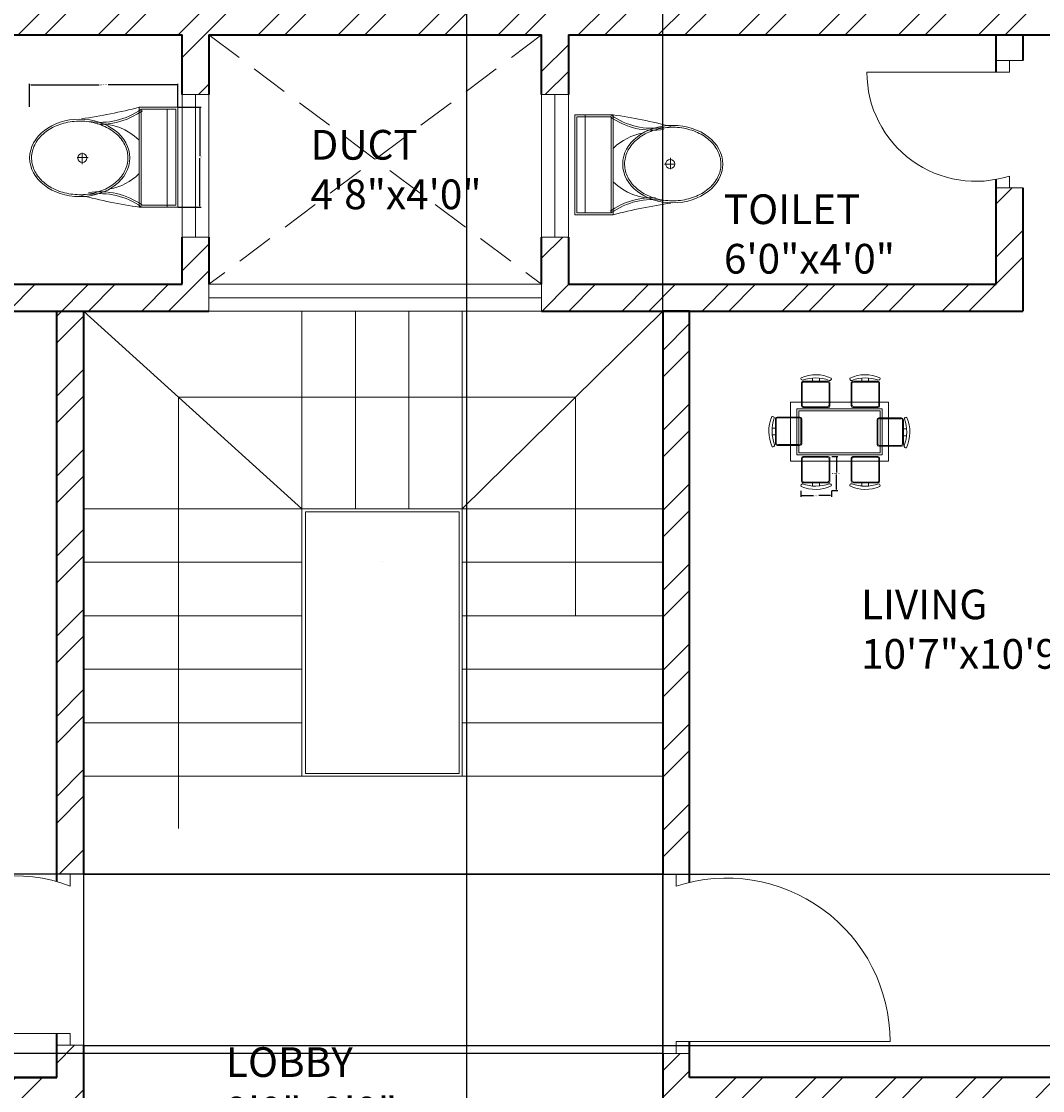
# Model space of a CAD drawing. Units: inches. Extents: x 1570 to 2186, y 1575 to 2421.
# Tile 8 of 10: x 1806 to 1978, y 2045 to 2225. Entities that reach past the tile are written whole.
import ezdxf

# ---------------------------------------------------------------- set-up
doc = ezdxf.new("R2010")
doc.units = ezdxf.units.IN
doc.linetypes.add('DASHED2', pattern=[9.525, 6.35, -3.175])
for name, color, linetype, lineweight in [('A-ANNO-DIMS', 2, 'Continuous', 18), ('A-AREA-IDEN', 7, 'Continuous', 18), ('A-DOOR', 201, 'Continuous', 18), ('A-FLOR-FIXT', 9, 'Continuous', 18), ('A-FLOR-OPEN', 254, 'DASHED2', 13), ('A-FLOR-STRS', 201, 'Continuous', 18), ('A-FURN', 8, 'Continuous', 13), ('A-GLAZ', 150, 'Continuous', 18), ('A-WALL', 7, 'Continuous', 35), ('A-WALL-PATT', 252, 'Continuous', 13)]:
    doc.layers.add(name, color=color, linetype=linetype, lineweight=lineweight)
doc.styles.get("Standard").update_dxf_attribs({"font": 'arial.ttf'})
doc.dimstyles.get("Standard").update_dxf_attribs({"dimtxt": 0.18, "dimasz": 0.18, "dimexe": 0.18, "dimexo": 0.0625, "dimgap": 0.09, "dimtad": 0, "dimtih": 1, "dimtoh": 1, "dimdec": 4, "dimzin": 0, "dimdsep": 46, "dimtxsty": 'Standard', "dimcen": 0.09, "dimadec": 0, "dimazin": 0, "dimtfac": 1, "dimtdec": 4, "dimtofl": 0, "dimtmove": 0, "dimatfit": 3, "dimfxl": 1, "dimtolj": 1, "dimtzin": 0, "dimarcsym": 0})

# ---------------------------------------------------------------- blocks, each defined once
blk = doc.blocks.new('A$C31115884')
for p, q in [((257.5, 466.4), (257.5, 523.2)), ((283.1, 497.7), (223.4, 497.7)), ((0, 200), (0, 0)), ((520, 200), (0, 200)), ((10, 190), (10, 10)), ((510, 190), (10, 190)), ((510, 10), (510, 190)), ((520, 0), (520, 200)), ((510, 54.5), (0, 54.5)), ((10, 10), (510, 10)), ((0, 0), (520, 0))]:
    blk.add_line(p, q)
blk.add_circle((255.6, 496.4), 23.6)
for centre, radius, start, end in [((2777.7, -204.6), 2807, 165.4549, 171.7133), ((-294.5, 403.3), 364.7, 324.2091, 9.3499), ((-294.5, 403.3), 374.7, 324.2091, 9.3499), ((805.8, 403.3), 364.7, 170.6501, 215.7909), ((3237, 905), 2807, 188.2867, 194.5451), ((139.5, 406.2), 293.5, 315.8436, 2.6563), ((805.8, 403.3), 374.7, 179.2036, 215.7909), ((383.6, 406.2), 293.5, 190.2774, 224.1564)]:
    blk.add_arc(centre, radius, start, end)
blk.add_ellipse((256.2, 509.9), major_axis=(0, -260.7), ratio=0.772727)
blk.add_open_spline([(256.2, 259.2), (263.1, 259.2), (270, 259.7), (287.8, 262.3), (298.7, 265.1), (319.9, 273.1), (330.2, 278.4), (350.1, 291.1), (359.7, 298.7), (377.7, 315.9), (386.2, 325.5), (401.7, 346.6), (408.8, 358.1), (421.3, 382.5), (426.8, 395.5), (435.9, 422.4), (439.5, 436.4), (444.8, 465.1), (446.5, 479.7), (447.9, 509.2), (447.6, 524), (445, 553.3), (442.7, 567.8), (436.3, 596), (432.1, 609.7), (421.9, 636), (416, 648.6), (402.5, 672.1), (395, 683), (378.6, 703), (369.8, 712.1), (351.1, 728), (341.3, 734.8), (320.9, 746.2), (310.4, 750.7), (288.9, 757.3), (278, 759.4), (256, 761), (245, 760.6), (223.1, 757.2), (212.3, 754.3), (191.1, 746.1), (180.8, 740.7), (160.9, 727.8), (151.4, 720.1), (133.5, 702.7), (125.1, 693), (109.6, 671.7), (102.6, 660.2), (90.2, 635.7), (84.9, 622.7), (76, 595.6), (72.4, 581.6), (67.2, 552.9), (65.6, 538.2), (64.4, 508.8), (64.8, 494), (67.5, 464.7), (69.9, 450.2), (76.6, 422), (80.8, 408.3), (91.1, 382.2), (97.2, 369.7), (110.8, 346.3), (118.4, 335.4), (134.8, 315.6), (143.7, 306.7), (162.4, 290.9), (172.3, 284.2), (192.8, 273), (203.3, 268.6), (224.8, 262.2), (235.8, 260.2), (249.9, 259.3), (253, 259.2), (256.2, 259.2)], degree=3, knots=[0, 0, 0, 0, 0.110105, 0.110105, 0.285049, 0.285049, 0.459994, 0.459994, 0.634938, 0.634938, 0.809882, 0.809882, 0.984827, 0.984827, 1.159771, 1.159771, 1.334715, 1.334715, 1.50966, 1.50966, 1.684604, 1.684604, 1.859549, 1.859549, 2.034493, 2.034493, 2.209437, 2.209437, 2.384382, 2.384382, 2.559326, 2.559326, 2.73427, 2.73427, 2.909215, 2.909215, 3.084159, 3.084159, 3.259103, 3.259103, 3.434048, 3.434048, 3.608992, 3.608992, 3.783936, 3.783936, 3.958881, 3.958881, 4.133825, 4.133825, 4.30877, 4.30877, 4.483714, 4.483714, 4.658658, 4.658658, 4.833603, 4.833603, 5.008547, 5.008547, 5.183491, 5.183491, 5.358436, 5.358436, 5.53338, 5.53338, 5.708324, 5.708324, 5.883269, 5.883269, 6.058213, 6.058213, 6.233158, 6.233158, 6.283185, 6.283185, 6.283185, 6.283185])
blk = doc.blocks.new('TABLE-DINING')
for points in [[(0, 9.93), (16.54, 9.93), (16.54, 0), (0, 0)], [(0, 9.93), (16.54, 9.93), (16.54, 0), (0, 0)], [(1.1, 8.82), (15.44, 8.82), (15.44, 1.1), (1.1, 1.1)], [(1.1, 8.82), (15.44, 8.82), (15.44, 1.1), (1.1, 1.1)], [(1.43, 8.49), (15.11, 8.49), (15.11, 1.43), (1.43, 1.43)], [(1.43, 8.49), (15.11, 8.49), (15.11, 1.43), (1.43, 1.43)]]:
    blk.add_lwpolyline(points, close=True)
blk = doc.blocks.new('WIN-24IN')
for p, q in [((2.25, 24), (0, 24)), ((0, 24), (4.5, 24)), ((0, 24), (0, 0)), ((2.25, 0), (2.25, 24)), ((4.5, 24), (4.5, 0)), ((0, 0), (4.5, 0)), ((4.5, 0), (2.25, 0))]:
    blk.add_line(p, q)
blk = doc.blocks.new('DINING-CHAIR-LH')
for points in [[(4.59, 1.1), (0.4, 1.1, -0.414214), (0.11, 1.39), (0.11, 5.24, -0.414214), (0.4, 5.53), (4.59, 5.53, -0.414214), (4.88, 5.24), (4.88, 1.39, -0.414214), (4.59, 1.1)], [(4.59, 1.1), (0.4, 1.1, -0.414214), (0.11, 1.39), (0.11, 5.24, -0.414214), (0.4, 5.53), (4.59, 5.53, -0.414214), (4.88, 5.24), (4.88, 1.39, -0.414214), (4.59, 1.1)], [(4.78, 0.96, -0.578392), (5.12, 0.58, -0.214524), (0.03, 0.51, -0.552014), (0.27, 0.92, 0.175809), (4.78, 0.96)], [(4.78, 0.96, -0.578392), (5.12, 0.58, -0.214524), (0.03, 0.51, -0.552014), (0.27, 0.92, 0.175809), (4.78, 0.96)], [(3.12, 1.1), (3.12, 0.57, 0.064759)], [(3.12, 1.1), (3.12, 0.57, 0.064759)]]:
    blk.add_lwpolyline(points, format="xyb")
blk.add_lwpolyline([(0.4, 1.23), (4.45, 1.23, 0.414214), (4.75, 1.53), (4.75, 5.11, 0.414214), (4.45, 5.4), (0.4, 5.4, 0.512069), (0.24, 5.11), (0.24, 1.53, 0.512069)], format="xyb", close=True)
blk.add_lwpolyline([(0.4, 1.23), (4.45, 1.23, 0.414214), (4.75, 1.53), (4.75, 5.11, 0.414214), (4.45, 5.4), (0.4, 5.4, 0.512069), (0.24, 5.11), (0.24, 1.53, 0.512069)], format="xyb", close=True)
blk.add_lwpolyline([(1.95, 0.56), (1.95, 1.1)])
blk.add_lwpolyline([(1.95, 0.56), (1.95, 1.1)])
blk = doc.blocks.new('*D12')
at = {"layer": 'A-ANNO-DIMS', "color": 0, "lineweight": -2, "transparency": 16777216}
for p, q in [((1807.02, 2210.52), (1807.02, 2214.38)), ((1807.2, 2214.2), (1818.71, 2214.2)), ((1831.77, 2214.2), (1820.26, 2214.2)), ((1831.95, 2210.52), (1831.95, 2214.38))]:
    blk.add_line(p, q, dxfattribs=at)
at = {"layer": 'A-ANNO-DIMS', "color": 0, "transparency": 16777216}
for points in [[(1807.2, 2214.23), (1807.2, 2214.17), (1807.02, 2214.2)], [(1831.77, 2214.23), (1831.77, 2214.17), (1831.95, 2214.2)]]:
    blk.add_solid(points, dxfattribs=at)
at = {"layer": 'Defpoints', "color": 0, "transparency": 16777216}
for p in [(1807.02, 2214.2), (1807.02, 2210.46), (1831.95, 2210.46)]:
    blk.add_point(p, dxfattribs=at)
at = {"layer": 'A-ANNO-DIMS', "color": 0, "transparency": 16777216, "insert": (1819.49, 2214.2), "char_height": 0.18, "attachment_point": 5}
blk.add_mtext('\\A1;WC 25 TYP.', dxfattribs=at)
blk = doc.blocks.new('*D13')
at = {"layer": 'A-ANNO-DIMS', "color": 0, "lineweight": -2, "transparency": 16777216}
for p, q in [((1832.01, 2210.46), (1835.87, 2210.46)), ((1835.69, 2210.28), (1835.69, 2202.23)), ((1835.69, 2193.82), (1835.69, 2201.87)), ((1832.01, 2193.64), (1835.87, 2193.64))]:
    blk.add_line(p, q, dxfattribs=at)
at = {"layer": 'A-ANNO-DIMS', "color": 0, "transparency": 16777216}
for points in [[(1835.66, 2210.28), (1835.72, 2210.28), (1835.69, 2210.46)], [(1835.66, 2193.82), (1835.72, 2193.82), (1835.69, 2193.64)]]:
    blk.add_solid(points, dxfattribs=at)
at = {"layer": 'Defpoints', "color": 0, "transparency": 16777216}
for p in [(1831.95, 2210.46), (1835.69, 2210.46), (1831.95, 2193.64)]:
    blk.add_point(p, dxfattribs=at)
at = {"layer": 'A-ANNO-DIMS', "color": 0, "transparency": 16777216, "insert": (1835.69, 2202.05), "char_height": 0.18, "attachment_point": 5}
blk.add_mtext('\\A1;17 TYP.', dxfattribs=at)
blk = doc.blocks.new('*D18')
at = {"layer": 'A-ANNO-DIMS', "color": 0, "lineweight": -2, "transparency": 16777216}
for p, q in [((1942.04, 2151.67), (1943.02, 2151.67)), ((1942.84, 2151.49), (1942.84, 2148.99)), ((1942.84, 2146.12), (1942.84, 2148.62)), ((1942.04, 2145.94), (1943.02, 2145.94))]:
    blk.add_line(p, q, dxfattribs=at)
at = {"layer": 'A-ANNO-DIMS', "color": 0, "transparency": 16777216}
for points in [[(1942.81, 2151.49), (1942.87, 2151.49), (1942.84, 2151.67)], [(1942.81, 2146.12), (1942.87, 2146.12), (1942.84, 2145.94)]]:
    blk.add_solid(points, dxfattribs=at)
at = {"layer": 'Defpoints', "color": 0, "transparency": 16777216}
for p in [(1941.98, 2151.67), (1942.84, 2151.67), (1941.98, 2145.94)]:
    blk.add_point(p, dxfattribs=at)
at = {"layer": 'A-ANNO-DIMS', "color": 0, "transparency": 16777216, "insert": (1942.84, 2148.8), "char_height": 0.18, "attachment_point": 5}
blk.add_mtext('\\A1;LH CHAIR 6 TYP.', dxfattribs=at)
blk = doc.blocks.new('*D19')
at = {"layer": 'A-ANNO-DIMS', "color": 0, "lineweight": -2, "transparency": 16777216}
for p, q in [((1936.81, 2145.88), (1936.81, 2144.9)), ((1936.99, 2145.08), (1938.94, 2145.08)), ((1941.8, 2145.08), (1939.85, 2145.08)), ((1941.98, 2145.88), (1941.98, 2144.9))]:
    blk.add_line(p, q, dxfattribs=at)
at = {"layer": 'A-ANNO-DIMS', "color": 0, "transparency": 16777216}
for points in [[(1936.99, 2145.11), (1936.99, 2145.05), (1936.81, 2145.08)], [(1941.8, 2145.11), (1941.8, 2145.05), (1941.98, 2145.08)]]:
    blk.add_solid(points, dxfattribs=at)
at = {"layer": 'Defpoints', "color": 0, "transparency": 16777216}
for p in [(1936.81, 2145.94), (1941.98, 2145.94), (1941.98, 2145.08)]:
    blk.add_point(p, dxfattribs=at)
at = {"layer": 'A-ANNO-DIMS', "color": 0, "transparency": 16777216, "insert": (1939.39, 2145.08), "char_height": 0.18, "attachment_point": 5}
blk.add_mtext('\\A1;5 TYP.', dxfattribs=at)
blk = doc.blocks.new('*D39')
at = {"layer": 'A-ANNO-DIMS', "color": 0, "lineweight": -2, "transparency": 16777216}
for p, q in [((1816.09, 2097.8), (1816.09, 1616.73)), ((1913.59, 2097.8), (1913.59, 1616.73)), ((1816.27, 1616.91), (1864.51, 1616.91)), ((1913.41, 1616.91), (1865.16, 1616.91))]:
    blk.add_line(p, q, dxfattribs=at)
at = {"layer": 'A-ANNO-DIMS', "color": 0, "transparency": 16777216}
for points in [[(1816.27, 1616.94), (1816.27, 1616.88), (1816.09, 1616.91)], [(1913.41, 1616.94), (1913.41, 1616.88), (1913.59, 1616.91)]]:
    blk.add_solid(points, dxfattribs=at)
at = {"layer": 'Defpoints', "color": 0, "transparency": 16777216}
for p in [(1816.09, 2097.86), (1913.59, 2097.86), (1913.59, 1616.91)]:
    blk.add_point(p, dxfattribs=at)
at = {"layer": 'A-ANNO-DIMS', "color": 0, "transparency": 16777216, "insert": (1864.84, 1616.91), "char_height": 0.18, "attachment_point": 5}
blk.add_mtext('\\A1;97.5', dxfattribs=at)
blk = doc.blocks.new('*D40')
at = {"layer": 'A-ANNO-DIMS', "color": 0, "lineweight": -2, "transparency": 16777216}
for p, q in [((1816.15, 2081.37), (2126.57, 2081.37)), ((2126.39, 2081.19), (2126.39, 2067.15)), ((2126.39, 2052.75), (2126.39, 2066.79)), ((1816.15, 2052.57), (2126.57, 2052.57))]:
    blk.add_line(p, q, dxfattribs=at)
at = {"layer": 'A-ANNO-DIMS', "color": 0, "transparency": 16777216}
for points in [[(2126.36, 2081.19), (2126.42, 2081.19), (2126.39, 2081.37)], [(2126.36, 2052.75), (2126.42, 2052.75), (2126.39, 2052.57)]]:
    blk.add_solid(points, dxfattribs=at)
at = {"layer": 'Defpoints', "color": 0, "transparency": 16777216}
for p in [(1816.09, 2081.37), (2126.39, 2081.37), (1816.09, 2052.57)]:
    blk.add_point(p, dxfattribs=at)
at = {"layer": 'A-ANNO-DIMS', "color": 0, "transparency": 16777216, "insert": (2126.39, 2066.97), "char_height": 0.18, "attachment_point": 5}
blk.add_mtext('\\A1;28.8', dxfattribs=at)
blk = doc.blocks.new('*D42')
at = {"layer": 'A-ANNO-DIMS', "color": 0, "lineweight": -2, "transparency": 16777216}
for p, q in [((1913.53, 2081.37), (1603.11, 2081.37)), ((1603.29, 2081.19), (1603.29, 2066.47)), ((1603.29, 2051.39), (1603.29, 2066.11)), ((1913.53, 2051.21), (1603.11, 2051.21))]:
    blk.add_line(p, q, dxfattribs=at)
at = {"layer": 'A-ANNO-DIMS', "color": 0, "transparency": 16777216}
for points in [[(1603.26, 2081.19), (1603.32, 2081.19), (1603.29, 2081.37)], [(1603.26, 2051.39), (1603.32, 2051.39), (1603.29, 2051.21)]]:
    blk.add_solid(points, dxfattribs=at)
at = {"layer": 'Defpoints', "color": 0, "transparency": 16777216}
for p in [(1603.29, 2081.37), (1913.59, 2081.37), (1913.59, 2051.21)]:
    blk.add_point(p, dxfattribs=at)
at = {"layer": 'A-ANNO-DIMS', "color": 0, "transparency": 16777216, "insert": (1603.29, 2066.29), "char_height": 0.18, "attachment_point": 5}
blk.add_mtext('\\A1;30.165', dxfattribs=at)
blk = doc.blocks.new('*D45')
at = {"layer": 'A-ANNO-DIMS', "color": 0, "lineweight": -2, "transparency": 16777216}
for p, q in [((1880.59, 1913.81), (1880.59, 2398.63)), ((1880.77, 2398.45), (1896.87, 2398.45)), ((1913.41, 2398.45), (1897.31, 2398.45)), ((1913.59, 1913.81), (1913.59, 2398.63))]:
    blk.add_line(p, q, dxfattribs=at)
at = {"layer": 'A-ANNO-DIMS', "color": 0, "transparency": 16777216}
for points in [[(1880.77, 2398.48), (1880.77, 2398.42), (1880.59, 2398.45)], [(1913.41, 2398.48), (1913.41, 2398.42), (1913.59, 2398.45)]]:
    blk.add_solid(points, dxfattribs=at)
at = {"layer": 'Defpoints', "color": 0, "transparency": 16777216}
for p in [(1913.59, 2398.45), (1880.59, 1913.75), (1913.59, 1913.75)]:
    blk.add_point(p, dxfattribs=at)
at = {"layer": 'A-ANNO-DIMS', "color": 0, "transparency": 16777216, "insert": (1897.09, 2398.45), "char_height": 0.18, "attachment_point": 5}
blk.add_mtext('\\A1;33', dxfattribs=at)

msp = doc.modelspace()

# ---------------------------------------------------------------- hatches: boundary and pattern name
at = {"layer": 'A-WALL-PATT'}
h = msp.add_hatch(dxfattribs=at)
h.set_pattern_fill('ANSI32', color=256)
h.paths.add_polyline_path([(1762.0975, 2362.1492), (1757.5975, 2362.1492), (1757.5975, 2357.6492), (1709.1163, 2357.6492), (1709.1163, 2362.1492), (1704.6163, 2362.1492), (1704.6163, 2353.1492), (1740.0886, 2353.1492), (1740.0886, 2261.8115), (1744.5886, 2261.8115), (1744.5886, 2353.1492), (1762.0975, 2353.1492)])
h.paths.add_polyline_path([(1890.2592, 2362.1492), (1885.7592, 2362.1492), (1826.5975, 2362.1492), (1822.0975, 2362.1492), (1822.0975, 2353.1492), (1862.5886, 2353.1492), (1862.5886, 2227.1492), (1744.5886, 2227.1492), (1744.5886, 2229.5389), (1742.3386, 2229.5389), (1740.0886, 2229.5389), (1740.0886, 2222.6492), (1744.5886, 2222.6492), (1756.186, 2222.6492), (1756.186, 2216.3571), (1760.686, 2216.3571), (1760.686, 2222.6492), (1832.686, 2222.6492), (1832.686, 2212.5994), (1837.186, 2212.5994), (1837.186, 2222.6492), (1893.186, 2222.6492), (1893.186, 2212.5994), (1897.686, 2212.5994), (1897.686, 2222.6492), (1989.5886, 2222.6492), (1989.5886, 2227.1492), (1989.5886, 2232.6585), (1987.3386, 2232.6585), (1985.0886, 2232.6585), (1985.0886, 2227.1492), (1867.0886, 2227.1492), (1867.0886, 2353.1492), (1890.2592, 2353.1492)])
h.paths.add_polyline_path([(1644.0886, 2353.1492), (1668.6163, 2353.1492), (1668.6163, 2362.1492), (1664.1163, 2362.1492), (1664.1163, 2358.9932), (1664.1163, 2357.6492), (1639.5886, 2357.6492), (1639.5886, 2213.8746), (1644.0886, 2213.8746), (1644.0886, 2222.6492), (1692.0886, 2222.6492), (1692.0886, 2215.9343), (1696.5886, 2215.9343), (1696.5886, 2222.6492), (1696.5886, 2227.1492), (1644.0886, 2227.1492)])
h.paths.add_polyline_path([(2013.0435, 2362.1492), (2008.5435, 2362.1492), (2008.5435, 2357.6492), (1954.7592, 2357.6492), (1954.7592, 2362.1492), (1950.2592, 2362.1492), (1950.2592, 2353.1492), (1985.0886, 2353.1492), (1985.0886, 2260.8534), (1989.5886, 2260.8534), (1989.5886, 2353.1492), (2013.0435, 2353.1492)])
h.paths.add_polyline_path([(2090.0886, 2357.6492), (2053.5435, 2357.6492), (2053.5435, 2362.1492), (2049.0435, 2362.1492), (2049.0435, 2353.1492), (2085.5886, 2353.1492), (2085.5886, 2227.1492), (2033.0886, 2227.1492), (2033.0886, 2222.6492), (2033.0886, 2214.4464), (2037.5886, 2214.4464), (2037.5886, 2222.6492), (2085.5886, 2222.6492), (2085.5886, 2212.4409), (2090.0886, 2212.4409)])
h.paths.add_polyline_path([(2090.0886, 2188.4409), (2087.8386, 2188.4409), (2085.5886, 2188.4409), (2085.5886, 2180.6492), (2037.5886, 2180.6492), (2037.5886, 2196.7956), (2033.0886, 2196.7956), (2033.0886, 2176.1492), (2037.5886, 2176.1492), (2045.0886, 2176.1492), (2045.0886, 2169.8988), (2049.5886, 2169.8988), (2049.5886, 2176.1492), (2085.5886, 2176.1492), (2085.5886, 2167.785), (2090.0886, 2167.785)])
h.paths.add_polyline_path([(2049.5886, 2147.4502), (2047.3386, 2147.4502), (2045.0886, 2147.4502), (2045.0886, 2124.4703), (2049.5886, 2124.4703)])
h.paths.add_polyline_path([(2090.0886, 2047.1492), (2049.5886, 2047.1492), (2049.5886, 2064.4703), (2045.0886, 2064.4703), (2045.0886, 2047.1492), (1918.0886, 2047.1492), (1918.0886, 2051.2061), (1913.5886, 2051.2061), (1913.5886, 2047.1492), (1913.5886, 2036.6872), (1918.0886, 2036.6872), (1918.0886, 2042.7492), (2045.0886, 2042.7492), (2045.0886, 2027.0686), (2049.5886, 2027.0686), (2049.5886, 2042.7492), (2090.0886, 2042.7492)])
h.paths.add_polyline_path([(1918.0886, 2005.9338), (1915.8386, 2005.9338), (1913.5886, 2005.9338), (1913.5886, 1913.7492), (1918.0886, 1913.7492)])
h.paths.add_polyline_path([(2090.0886, 1913.7492), (2049.5886, 1913.7492), (2045.0886, 1913.7492), (2033.0886, 1913.7492), (2033.0886, 1909.2492), (2033.0886, 1900.9803), (2037.5886, 1900.9803), (2037.5886, 1909.2492), (2085.5886, 1909.2492), (2085.5886, 1861.2492), (2037.5886, 1861.2492), (2037.5886, 1880.0859), (2033.0886, 1880.0859), (2033.0886, 1856.7492), (2085.5886, 1856.7492), (2085.5886, 1730.7492), (2054.2483, 1730.7492), (2054.2483, 1721.7492), (2058.7483, 1721.7492), (2058.7483, 1726.2492), (2090.0886, 1726.2492)])
h.paths.add_polyline_path([(2049.5886, 1967.0686), (2045.0886, 1967.0686), (2045.0886, 1913.7492), (2049.5886, 1913.7492)])
h.paths.add_polyline_path([(1989.5886, 1824.1695), (1987.3386, 1824.1695), (1985.0886, 1824.1695), (1985.0886, 1730.7492), (1989.5886, 1730.7492)])
h.paths.add_polyline_path([(1989.5886, 1861.2492), (1974.9963, 1861.2492), (1974.9963, 1865.9306), (1972.7463, 1865.9306), (1970.4963, 1865.9306), (1970.4963, 1861.2492), (1898.4963, 1861.2492), (1898.4963, 1874.2999), (1893.9963, 1874.2999), (1893.9963, 1861.2492), (1890.5886, 1861.2492), (1837.9963, 1861.2492), (1837.9963, 1874.3159), (1833.4963, 1874.3159), (1833.4963, 1861.2492), (1761.4963, 1861.2492), (1761.4963, 1865.0209), (1759.2463, 1865.0209), (1756.9963, 1865.0209), (1756.9963, 1861.2492), (1740.0886, 1861.2492), (1740.0886, 1856.7492), (1740.0886, 1850.7206), (1744.5886, 1850.7206), (1744.5886, 1856.7492), (1985.0886, 1856.7492), (1985.0886, 1851.0804), (1989.5886, 1851.0804), (1989.5886, 1856.7492)])
h.paths.add_polyline_path([(1989.5886, 1913.7492), (1740.0886, 1913.7492), (1740.0886, 1909.2492), (1756.9963, 1909.2492), (1756.9963, 1890.279), (1761.4963, 1890.279), (1761.4963, 1909.2492), (1833.4963, 1909.2492), (1833.4963, 1898.3159), (1837.9963, 1898.3159), (1837.9963, 1909.2492), (1890.5886, 1909.2492), (1893.9963, 1909.2492), (1893.9963, 1898.2999), (1898.4963, 1898.2999), (1898.4963, 1909.2492), (1970.4963, 1909.2492), (1970.4963, 1886.9887), (1974.9963, 1886.9887), (1974.9963, 1909.2492), (1989.5886, 1909.2492)])
h.paths.add_polyline_path([(1893.7344, 1730.7492), (1867.0886, 1730.7492), (1867.0886, 1856.7492), (1862.5886, 1856.7492), (1862.5886, 1730.7492), (1824.0492, 1730.7492), (1824.0492, 1721.7492), (1893.7344, 1721.7492)])
h.paths.add_polyline_path([(2018.2483, 1730.7492), (1953.7344, 1730.7492), (1953.7344, 1721.7492), (1958.2344, 1721.7492), (1958.2344, 1726.2492), (2013.7483, 1726.2492), (2013.7483, 1721.7492), (2018.2483, 1721.7492)])
h.paths.add_polyline_path([(1768.5492, 1730.7492), (1764.0492, 1730.7492), (1744.5886, 1730.7492), (1744.5886, 1819.4364), (1742.3386, 1819.4364), (1740.0886, 1819.4364), (1740.0886, 1730.7492), (1697.3801, 1730.7492), (1697.3801, 1721.7492), (1701.8801, 1721.7492), (1701.8801, 1726.2492), (1764.0492, 1726.2492), (1764.0492, 1721.7492), (1768.5492, 1721.7492)])
h.paths.add_polyline_path([(1644.0886, 1856.7492), (1639.5886, 1856.7492), (1639.5886, 1726.2492), (1657.0315, 1726.2492), (1657.0315, 1721.7492), (1661.3801, 1721.7492), (1661.3801, 1730.7492), (1644.0886, 1730.7492)])
h.paths.add_polyline_path([(1696.5886, 1876.1809), (1692.0886, 1876.1809), (1692.0886, 1861.2492), (1684.5886, 1861.2492), (1644.0886, 1861.2492), (1644.0886, 1909.2492), (1692.0886, 1909.2492), (1692.0886, 1900.3394), (1696.5886, 1900.3394), (1696.5886, 1913.7492), (1684.5886, 1913.7492), (1684.5886, 1920.2115), (1682.3386, 1920.2115), (1680.0886, 1920.2115), (1680.0886, 1913.7492), (1639.5886, 1913.7492), (1639.5886, 1856.7492), (1684.5886, 1856.7492), (1692.0886, 1856.7492), (1696.5886, 1856.7492)])
h.paths.add_polyline_path([(1684.5886, 2042.7492), (1811.5886, 2042.7492), (1811.5886, 2038.2991), (1816.0886, 2038.2991), (1816.0886, 2042.7492), (1816.0886, 2052.5708), (1813.8386, 2052.5708), (1811.5886, 2052.5708), (1811.5886, 2047.1492), (1684.5886, 2047.1492), (1684.5886, 2064.4703), (1680.0886, 2064.4703), (1680.0886, 2047.1492), (1639.5886, 2047.1492), (1639.5886, 2042.7492), (1680.0886, 2042.7492), (1680.0886, 2024.0762), (1684.5886, 2024.0762)])
h.paths.add_polyline_path([(1684.5886, 1964.0762), (1680.0886, 1964.0762), (1680.0886, 1944.6145), (1684.5886, 1944.6145)])
h.paths.add_polyline_path([(1816.0886, 1973.7492), (1876.0886, 1973.7492), (1876.0886, 1959.17), (1880.5886, 1959.17), (1880.5886, 1973.7492), (1880.5886, 1978.2492), (1816.0886, 1978.2492), (1816.0886, 2005.9338), (1813.8386, 2005.9338), (1811.5886, 2005.9338), (1811.5886, 1913.7492), (1816.0886, 1913.7492)])
h.paths.add_polyline_path([(1837.186, 2180.6492), (1837.186, 2188.5994), (1834.936, 2188.5994), (1832.686, 2188.5994), (1832.686, 2180.6492), (1760.686, 2180.6492), (1760.686, 2197.4807), (1756.186, 2197.4807), (1756.186, 2180.6492), (1744.5886, 2180.6492), (1740.0886, 2180.6492), (1740.0886, 2176.1492), (1837.186, 2176.1492)])
h.paths.add_polyline_path([(1974.186, 2196.8744), (1971.936, 2196.8744), (1969.686, 2196.8744), (1969.686, 2180.6492), (1897.686, 2180.6492), (1897.686, 2188.5994), (1895.436, 2188.5994), (1893.186, 2188.5994), (1893.186, 2180.6492), (1893.186, 2176.1492), (1974.186, 2176.1492)])
h.paths.add_polyline_path([(1918.0886, 2176.1492), (1913.5886, 2176.1492), (1913.5886, 2081.3709), (1918.0886, 2081.3709)])
h.paths.add_polyline_path([(1816.0886, 2176.1492), (1811.5886, 2176.1492), (1811.5886, 2081.3709), (1816.0886, 2081.3709)])
h.paths.add_polyline_path([(1684.5886, 2150.4939), (1682.3386, 2150.4939), (1680.0886, 2150.4939), (1680.0886, 2124.4703), (1684.5886, 2124.4703)])
h.paths.add_polyline_path([(1696.5886, 2180.6492), (1696.5886, 2197.4701), (1692.0886, 2197.4701), (1692.0886, 2180.6492), (1644.0886, 2180.6492), (1644.0886, 2189.8746), (1641.8386, 2189.8746), (1639.5886, 2189.8746), (1639.5886, 2169.814), (1644.0886, 2169.814), (1644.0886, 2176.1492), (1680.0886, 2176.1492), (1680.0886, 2171.7002), (1684.5886, 2171.7002), (1684.5886, 2176.1492), (1696.5886, 2176.1492)])

# ---------------------------------------------------------------- linework, layer by layer
at = {"layer": 'A-DOOR'}
for p, q in [((1974.186, 2218.3349), (1969.686, 2218.3349)), ((1969.686, 2218.3349), (1971.936, 2218.3349)), ((1971.936, 2218.3349), (1971.936, 2216.3349)), ((1971.936, 2216.3349), (1947.936, 2216.3349)), ((1971.936, 2196.8744), (1971.936, 2198.8744)), ((1969.686, 2196.8744), (1974.186, 2196.8744)), ((1974.186, 2196.8744), (1971.936, 2196.8744)), ((1811.5886, 2081.3709), (1816.0886, 2081.3709)), ((1816.0886, 2081.3709), (1813.8386, 2081.3709)), ((1813.8386, 2081.3709), (1813.8386, 2079.3709)), ((1913.5886, 2081.3709), (1918.0886, 2081.3709)), ((1918.0886, 2081.3709), (1915.8386, 2081.3709)), ((1915.8386, 2081.3709), (1915.8386, 2079.3709)), ((1813.8386, 2054.5708), (1777.8386, 2054.5708)), ((1813.8386, 2052.5708), (1813.8386, 2054.5708)), ((1811.5886, 2052.5708), (1816.0886, 2052.5708)), ((1816.0886, 2052.5708), (1813.8386, 2052.5708)), ((1915.8386, 2051.2061), (1915.8386, 2053.2061)), ((1915.8386, 2053.2061), (1951.8386, 2053.2061)), ((1918.0886, 2051.2061), (1913.5886, 2051.2061)), ((1913.5886, 2051.2061), (1915.8386, 2051.2061))]:
    msp.add_line(p, q, dxfattribs=at)
for centre, radius, start, end in [((1966.2874, 2216.3349), 18.3514, 180, 287.926685), ((1804.381, 2054.5708), 26.5423, 69.125341, 180), ((1924.3303, 2053.2061), 27.5083, 360, 107.980576)]:
    msp.add_arc(centre, radius, start, end, dxfattribs=at)
at = {"layer": 'A-FLOR-OPEN'}
for p, q in [((1893.186, 2222.6492), (1837.186, 2180.6492)), ((1837.186, 2222.6492), (1893.186, 2180.6492))]:
    msp.add_line(p, q, dxfattribs=at)
at = {"layer": 'A-FLOR-STRS'}
for p, q in [((1852.8386, 2142.8597), (1816.0886, 2176.1492)), ((1852.8386, 2142.8597), (1852.8386, 2176.1492)), ((1861.8386, 2142.8597), (1861.8386, 2176.1492)), ((1870.8386, 2142.8597), (1870.8386, 2176.1492)), ((1879.8386, 2142.8597), (1879.8386, 2176.1492)), ((1879.8386, 2142.8597), (1913.5886, 2176.1492)), ((1832.073, 2161.6699), (1898.9195, 2161.6802)), ((1832.0956, 2089.085), (1832.073, 2161.6699)), ((1898.9195, 2161.6802), (1898.9195, 2124.8597)), ((1816.0886, 2142.8597), (1913.5886, 2142.8597)), ((1852.8386, 2142.8597), (1852.8386, 2097.8597)), ((1853.4482, 2142.3695), (1879.2846, 2142.3695)), ((1879.8386, 2142.8597), (1879.8386, 2097.8597)), ((1816.0886, 2133.8597), (1852.8386, 2133.8597)), ((1866.4293, 2133.9447), (1866.4293, 2133.9447)), ((1879.8386, 2133.8597), (1913.5886, 2133.8597)), ((1816.0886, 2124.8597), (1852.8386, 2124.8597)), ((1879.8386, 2124.8597), (1913.5886, 2124.8597)), ((1816.0886, 2115.8597), (1852.8386, 2115.8597)), ((1879.8386, 2115.8597), (1913.5886, 2115.8597)), ((1816.0886, 2106.8597), (1852.8386, 2106.8597)), ((1879.8386, 2106.8597), (1913.5886, 2106.8597)), ((1816.0886, 2097.8597), (1913.5886, 2097.8597)), ((1864.8386, 2097.8597), (1852.8386, 2097.8597))]:
    msp.add_line(p, q, dxfattribs=at)
msp.add_lwpolyline([(1879.2846, 2142.3695), (1879.2846, 2098.3419), (1853.4482, 2098.3419), (1853.4482, 2142.3695)], dxfattribs=at)
at = {"layer": 'A-FURN'}
for points in [[(1937.0968, 2164.5142, -0.17580919), (1941.6026, 2164.4801, 0.57839206), (1941.944, 2164.8555, 0.21452438), (1936.8578, 2164.9237, 0.55201397), (1937.0968, 2164.5142, -0.06507904)], [(1937.0968, 2164.5141, -0.17580919), (1941.6026, 2164.4799, 0.57839206), (1941.944, 2164.8553, 0.21452438), (1936.8578, 2164.9235, 0.55201397), (1937.0968, 2164.5141, -0.06507904)], [(1939.9421, 2164.3334), (1939.9421, 2164.8624, -0.06475861)], [(1939.9422, 2164.3332), (1939.9422, 2164.8623, -0.06475861)], [(1945.3959, 2164.4801, -0.57839206), (1945.0546, 2164.8555, -0.21452438), (1950.1407, 2164.9237, -0.55201397), (1949.9018, 2164.5142, 0.1758092), (1945.3959, 2164.4801)], [(1945.3959, 2164.4799, -0.57839206), (1945.0546, 2164.8553, -0.21452438), (1950.1407, 2164.9235, -0.55201397), (1949.9018, 2164.5141, 0.1758092), (1945.3959, 2164.4799)], [(1947.0564, 2164.3334), (1947.0564, 2164.8624, 0.06475861)], [(1947.0564, 2164.3332), (1947.0564, 2164.8623, 0.06475861)], [(1941.4114, 2164.3334), (1937.2284, 2164.3334, 0.41421356), (1936.9357, 2164.0407), (1936.9357, 2160.1945, 0.41421356), (1937.2284, 2159.9019), (1941.4114, 2159.9019, 0.41421356), (1941.7041, 2160.1945), (1941.7041, 2164.0407, 0.41421356), (1941.4114, 2164.3334)], [(1941.4115, 2164.3332), (1937.2284, 2164.3332, 0.41421356), (1936.9357, 2164.0406), (1936.9357, 2160.1943, 0.41421356), (1937.2284, 2159.9017), (1941.4115, 2159.9017, 0.41421356), (1941.7041, 2160.1943), (1941.7041, 2164.0406, 0.41421356), (1941.4115, 2164.3332)], [(1949.7701, 2164.3334, -0.41421356), (1950.0628, 2164.0407), (1950.0628, 2160.1945, -0.41421356), (1949.7701, 2159.9019), (1945.5871, 2159.9019, -0.41421356), (1945.2944, 2160.1945), (1945.2944, 2164.0407, -0.41421356), (1945.5871, 2164.3334), (1949.7701, 2164.3334)], [(1949.7702, 2164.3332, -0.41421356), (1950.0628, 2164.0406), (1950.0628, 2160.1943, -0.41421356), (1949.7702, 2159.9017), (1945.5871, 2159.9017, -0.41421356), (1945.2945, 2160.1943), (1945.2945, 2164.0406, -0.41421356), (1945.5871, 2164.3332), (1949.7702, 2164.3332)], [(1932.3828, 2153.6334, -0.57839206), (1932.0075, 2153.292, -0.21452438), (1931.9392, 2158.3781, -0.55201397), (1932.3487, 2158.1392, 0.17580937), (1932.3828, 2153.6334)], [(1932.3828, 2153.6332, -0.57839206), (1932.0075, 2153.2918, -0.21452438), (1931.9392, 2158.378, -0.55201397), (1932.3487, 2158.139, 0.17580937), (1932.3828, 2153.6332)], [(1932.5295, 2158.0076, -0.41421356), (1932.8222, 2158.3002), (1936.6684, 2158.3002, -0.41421356), (1936.9611, 2158.0076), (1936.9611, 2153.8245, -0.41421356), (1936.6684, 2153.5319), (1932.8222, 2153.5319, -0.41421356), (1932.5295, 2153.8245), (1932.5295, 2158.0076)], [(1932.5296, 2158.0074, -0.41421356), (1932.8222, 2158.3001), (1936.6684, 2158.3001, -0.41421356), (1936.9611, 2158.0074), (1936.9611, 2153.8243, -0.41421356), (1936.6684, 2153.5317), (1932.8222, 2153.5317, -0.41421356), (1932.5296, 2153.8243), (1932.5296, 2158.0074)], [(1954.0703, 2157.8643, 0.41421356), (1953.7777, 2158.157), (1949.9314, 2158.157, 0.41421356), (1949.6388, 2157.8643), (1949.6388, 2153.6813, 0.41421356), (1949.9314, 2153.3886), (1953.7777, 2153.3886, 0.41421356), (1954.0703, 2153.6813), (1954.0703, 2157.8643)], [(1954.0703, 2157.8641, 0.41421356), (1953.7777, 2158.1568), (1949.9314, 2158.1568, 0.41421356), (1949.6388, 2157.8641), (1949.6388, 2153.6811, 0.41421356), (1949.9314, 2153.3884), (1953.7777, 2153.3884, 0.41421356), (1954.0703, 2153.6811), (1954.0703, 2157.8641)], [(1954.2512, 2157.9959, -0.17580919), (1954.217, 2153.4901, 0.57839206), (1954.5924, 2153.1487, 0.21452438), (1954.6606, 2158.2349, 0.55201397), (1954.2512, 2157.9959, -0.06507904)], [(1954.2512, 2157.9957, -0.17580919), (1954.2171, 2153.4899, 0.57839206), (1954.5924, 2153.1486, 0.21452438), (1954.6606, 2158.2347, 0.55201397), (1954.2512, 2157.9958, -0.06507904)], [(1932.5295, 2155.2938), (1932.0005, 2155.2938, 0.06475861)], [(1932.5296, 2155.2936), (1932.0005, 2155.2936, 0.06475861)], [(1954.0703, 2155.1506), (1954.5994, 2155.1506, -0.06475861)], [(1954.0703, 2155.1504), (1954.5994, 2155.1504, -0.06475861)], [(1949.7701, 2147.2359, 0.41421356), (1950.0628, 2147.5286), (1950.0628, 2151.3748, 0.41421356), (1949.7701, 2151.6675), (1945.5871, 2151.6675, 0.41421356), (1945.2944, 2151.3748), (1945.2944, 2147.5286, 0.41421356), (1945.5871, 2147.2359), (1949.7701, 2147.2359)], [(1949.7702, 2147.2358, 0.41421356), (1950.0628, 2147.5284), (1950.0628, 2151.3746, 0.41421356), (1949.7702, 2151.6673), (1945.5871, 2151.6673, 0.41421356), (1945.2945, 2151.3746), (1945.2945, 2147.5284, 0.41421356), (1945.5871, 2147.2358), (1949.7702, 2147.2358)], [(1949.9018, 2147.0551, -0.17580928), (1945.3959, 2147.0892, 0.57839206), (1945.0546, 2146.7139, 0.21452438), (1950.1407, 2146.6456, 0.55201397), (1949.9018, 2147.0551, -0.06507904)], [(1949.9018, 2147.0549, -0.17580928), (1945.3959, 2147.089, 0.57839206), (1945.0546, 2146.7137, 0.21452438), (1950.1407, 2146.6454, 0.55201397), (1949.9018, 2147.0549, -0.06507904)], [(1947.0564, 2147.2359), (1947.0564, 2146.7069, -0.06475861)], [(1947.0564, 2147.2358), (1947.0564, 2146.7067, -0.06475861)]]:
    msp.add_lwpolyline(points, format="xyb", dxfattribs=at)
for points in [[(1938.7712, 2164.872), (1938.7712, 2164.3334)], [(1938.7713, 2164.8719), (1938.7713, 2164.3332)], [(1948.2273, 2164.872), (1948.2273, 2164.3334)], [(1948.2273, 2164.8719), (1948.2273, 2164.3332)], [(1931.9909, 2156.4647), (1932.5295, 2156.4647)], [(1931.9909, 2156.4645), (1932.5296, 2156.4645)], [(1954.609, 2156.3215), (1954.0703, 2156.3215)], [(1954.609, 2156.3213), (1954.0703, 2156.3213)], [(1948.2273, 2146.6973), (1948.2273, 2147.2359)], [(1948.2273, 2146.6971), (1948.2273, 2147.2358)]]:
    msp.add_lwpolyline(points, dxfattribs=at)
for points in [[(1937.2302, 2164.2016), (1941.2796, 2164.2016, -0.41421356), (1941.5723, 2163.9089), (1941.5723, 2160.3264, -0.41421356), (1941.2796, 2160.0337), (1937.2302, 2160.0337, -0.51206948), (1937.0676, 2160.3264), (1937.0676, 2163.9089, -0.51206948)], [(1937.2302, 2164.2014), (1941.2796, 2164.2014, -0.41421356), (1941.5723, 2163.9087), (1941.5723, 2160.3262, -0.41421356), (1941.2796, 2160.0335), (1937.2302, 2160.0335, -0.51206948), (1937.0676, 2160.3262), (1937.0676, 2163.9087, -0.51206948)], [(1949.7684, 2164.2016), (1945.7189, 2164.2016, 0.41421356), (1945.4263, 2163.9089), (1945.4263, 2160.3264, 0.41421356), (1945.7189, 2160.0337), (1949.7684, 2160.0337, 0.51206948), (1949.931, 2160.3264), (1949.931, 2163.9089, 0.51206948)], [(1949.7684, 2164.2014), (1945.7189, 2164.2014, 0.41421356), (1945.4263, 2163.9087), (1945.4263, 2160.3262, 0.41421356), (1945.7189, 2160.0335), (1949.7684, 2160.0335, 0.51206948), (1949.931, 2160.3262), (1949.931, 2163.9087, 0.51206948)], [(1932.6614, 2158.0058), (1932.6614, 2153.9564, 0.41421356), (1932.954, 2153.6637), (1936.5366, 2153.6637, 0.41421356), (1936.8292, 2153.9564), (1936.8292, 2158.0058, 0.51206948), (1936.5366, 2158.1684), (1932.954, 2158.1684, 0.51206948)], [(1932.6614, 2158.0056), (1932.6614, 2153.9562, 0.41421356), (1932.954, 2153.6635), (1936.5366, 2153.6635, 0.41421356), (1936.8293, 2153.9562), (1936.8293, 2158.0056, 0.51206948), (1936.5366, 2158.1682), (1932.954, 2158.1682, 0.51206948)], [(1953.9385, 2157.8625), (1953.9385, 2153.8131, -0.41421356), (1953.6458, 2153.5205), (1950.0633, 2153.5205, -0.41421356), (1949.7706, 2153.8131), (1949.7706, 2157.8625, -0.51206948), (1950.0633, 2158.0251), (1953.6458, 2158.0251, -0.51206948)], [(1953.9385, 2157.8624), (1953.9385, 2153.8129, -0.41421356), (1953.6458, 2153.5203), (1950.0633, 2153.5203, -0.41421356), (1949.7706, 2153.8129), (1949.7706, 2157.8624, -0.51206948), (1950.0633, 2158.025), (1953.6458, 2158.025, -0.51206948)], [(1949.7684, 2147.3678), (1945.7189, 2147.3678, -0.41421356), (1945.4263, 2147.6604), (1945.4263, 2151.243, -0.41421356), (1945.7189, 2151.5356), (1949.7684, 2151.5356, -0.51206948), (1949.931, 2151.243), (1949.931, 2147.6604, -0.51206948)], [(1949.7684, 2147.3676), (1945.7189, 2147.3676, -0.41421356), (1945.4263, 2147.6602), (1945.4263, 2151.2428, -0.41421356), (1945.7189, 2151.5355), (1949.7684, 2151.5355, -0.51206948), (1949.931, 2151.2428), (1949.931, 2147.6602, -0.51206948)]]:
    msp.add_lwpolyline(points, format="xyb", close=True, dxfattribs=at)
at = {"layer": 'A-GLAZ'}
for p, q in [((1837.186, 2180.6492), (1837.186, 2176.1492)), ((1837.186, 2180.6492), (1893.186, 2180.6492)), ((1893.186, 2180.6492), (1893.186, 2176.1492)), ((1893.186, 2178.3992), (1837.186, 2178.3992)), ((1837.186, 2176.1492), (1893.186, 2176.1492))]:
    msp.add_line(p, q, dxfattribs=at)
at = {"layer": 'A-WALL'}
for p, q in [((1760.686, 2222.6492), (1832.686, 2222.6492)), ((1832.686, 2212.5994), (1832.686, 2222.6492)), ((1837.186, 2222.6492), (1837.186, 2212.5994)), ((1837.186, 2222.6492), (1893.186, 2222.6492)), ((1893.186, 2212.5994), (1893.186, 2222.6492)), ((1897.686, 2222.6492), (1897.686, 2212.5994)), ((1897.686, 2222.6492), (1989.5886, 2222.6492)), ((1969.686, 2222.6492), (1974.186, 2222.6492)), ((1969.686, 2216.3349), (1969.686, 2222.6492)), ((1974.186, 2222.6492), (1974.186, 2218.3349)), ((1969.686, 2180.6492), (1969.686, 2198.3009)), ((1974.186, 2196.8744), (1974.186, 2176.1492)), ((1832.686, 2180.6492), (1832.686, 2188.5994)), ((1837.186, 2188.5994), (1837.186, 2180.6492)), ((1893.186, 2180.6492), (1893.186, 2188.5994)), ((1897.686, 2188.5994), (1897.686, 2180.6492)), ((1760.686, 2180.6492), (1832.686, 2180.6492)), ((1897.686, 2180.6492), (1969.686, 2180.6492)), ((1740.0886, 2176.1492), (1837.186, 2176.1492)), ((1811.5886, 2176.1492), (1816.0886, 2176.1492)), ((1811.5886, 2080.1157), (1811.5886, 2176.1492)), ((1816.0886, 2176.1492), (1816.0886, 2081.3709)), ((1893.186, 2176.1492), (1974.186, 2176.1492)), ((1918.0886, 2176.1492), (1913.5886, 2176.1492)), ((1913.5886, 2176.1492), (1913.5886, 2081.3709)), ((1918.0886, 2079.9969), (1918.0886, 2176.1492)), ((1811.5886, 2047.1492), (1811.5886, 2054.5708)), ((1816.0886, 2052.5708), (1816.0886, 2042.7492)), ((1918.0886, 2047.1492), (1918.0886, 2053.2061)), ((1913.5886, 2051.2061), (1913.5886, 2047.1492)), ((1684.5886, 2047.1492), (1811.5886, 2047.1492)), ((1811.5886, 2047.1492), (1684.5886, 2047.1492)), ((1913.5886, 2047.1492), (1913.5886, 2036.6872)), ((2045.0886, 2047.1492), (1918.0886, 2047.1492)), ((2045.0886, 2047.1492), (1918.0886, 2047.1492))]:
    msp.add_line(p, q, dxfattribs=at)

# ---------------------------------------------------------------- block references
at = {"layer": 'A-FLOR-FIXT', "xscale": 0.0323450304620732, "yscale": 0.0323450304620732, "zscale": 0.0323450304620732}
for p, rotation in [((1831.9488, 2193.6374), 89.99999999999996), ((1898.7717, 2209.1715), 269.9999999999999)]:
    msp.add_blockref('A$C31115884', p, dxfattribs=dict(at, rotation=rotation))
at = {"layer": 'A-FURN'}
for name, p in [('TABLE-DINING', (1935.0502, 2150.8748)), ('DINING-CHAIR-LH', (1936.8262, 2146.1338))]:
    msp.add_blockref(name, p, dxfattribs=at)
at = {"layer": 'A-GLAZ'}
for p in [(1832.6863, 2188.5995), (1893.1863, 2188.5995)]:
    msp.add_blockref('WIN-24IN', p, dxfattribs=at)

# ---------------------------------------------------------------- texts
at = {"layer": 'A-AREA-IDEN', "char_height": 5, "attachment_point": 1}
for s, width, insert in [('DUCT\\P4\'8"x4\'0"', 82.45476, (1854.2852, 2206.6255)), ('TOILET\\P6\'0"x4\'0"', 94.15963, (1923.8667, 2195.7866)), ('LIVING\\P10\'7"x10\'9"', 308.463782, (1946.9462, 2129.2788)), ('LOBBY\\P9\'0"x9\'0"', 115.828202, (1840.0646, 2052.2484))]:
    msp.add_mtext_dynamic_manual_height_columns(s, width=width, gutter_width=12.5, heights=[0], dxfattribs=dict(at, insert=insert))

# ---------------------------------------------------------------- dimensions: what is measured, and where the dimension line sits
at = {"layer": 'A-ANNO-DIMS'}
for base, p1, p2, override, picture, middle in [((1913.5886, 2398.4492), (1880.5886, 1913.7492), (1913.5886, 1913.7492), {"dimdec": 0, "dimlfac": 1, "dimrnd": 0, "dimzin": 0, "dimdsep": 46, "dimlunit": 2}, '*D45', (1897.0886, 2398.4492)), ((1913.5886, 1616.9104), (1816.0886, 2097.8597), (1913.5886, 2097.8597), {"dimdec": 1, "dimlfac": 1, "dimrnd": 0, "dimzin": 0, "dimdsep": 46, "dimlunit": 2}, '*D39', (1864.8386, 1616.9104))]:
    dim = msp.add_linear_dim(base=base, p1=p1, p2=p2, dimstyle='Standard', override=override, dxfattribs=at)
    dim.commit()
    dim.dimension.update_dxf_attribs({"geometry": picture, "text_midpoint": middle})
for base, p1, p2, angle, text, picture, middle in [((1807.0247, 2214.1954), (1831.9488, 2210.4568), (1807.0247, 2210.4568), 180, 'WC <> TYP.', '*D12', (1819.4867, 2214.1954)), ((1835.6874, 2210.4568), (1831.9488, 2193.6374), (1831.9488, 2210.4568), 90, '<> TYP.', '*D13', (1835.6874, 2202.0471)), ((1942.8351, 2151.6675), (1941.976, 2145.9397), (1941.976, 2151.6675), 90, 'LH CHAIR <> TYP.', '*D18', (1942.8351, 2148.8036))]:
    dim = msp.add_linear_dim(base=base, p1=p1, p2=p2, angle=angle, text=text, dimstyle='Standard', override={"dimdec": 0, "dimlfac": 1, "dimrnd": 0, "dimzin": 0, "dimdsep": 46, "dimlunit": 2}, dxfattribs=at)
    dim.commit()
    dim.dimension.update_dxf_attribs({"geometry": picture, "text_midpoint": middle})
dim = msp.add_linear_dim(base=(1941.976, 2145.0806), p1=(1936.8133, 2145.9397), p2=(1941.976, 2145.9397), text='<> TYP.', dimstyle='Standard', override={"dimdec": 0, "dimlfac": 1, "dimrnd": 0, "dimzin": 0, "dimdsep": 46, "dimlunit": 2}, dxfattribs=at)
dim.commit()
dim.dimension.update_dxf_attribs({"geometry": '*D19', "text_midpoint": (1939.3947, 2145.0806)})
for base, p1, p2, override, picture, middle in [((1603.2886, 2081.3709), (1913.5886, 2051.2061), (1913.5886, 2081.3709), {"dimdec": 3, "dimlfac": 1, "dimrnd": 0, "dimzin": 0, "dimdsep": 46, "dimlunit": 2}, '*D42', (1603.2886, 2066.2885)), ((2126.3886, 2081.3709), (1816.0886, 2052.5708), (1816.0886, 2081.3709), {"dimdec": 1, "dimlfac": 1, "dimrnd": 0, "dimzin": 0, "dimdsep": 46, "dimlunit": 2}, '*D40', (2126.3886, 2066.9709))]:
    dim = msp.add_linear_dim(base=base, p1=p1, p2=p2, angle=90, dimstyle='Standard', override=override, dxfattribs=at)
    dim.commit()
    dim.dimension.update_dxf_attribs({"geometry": picture, "text_midpoint": middle})

doc.saveas('drawing.dxf')
